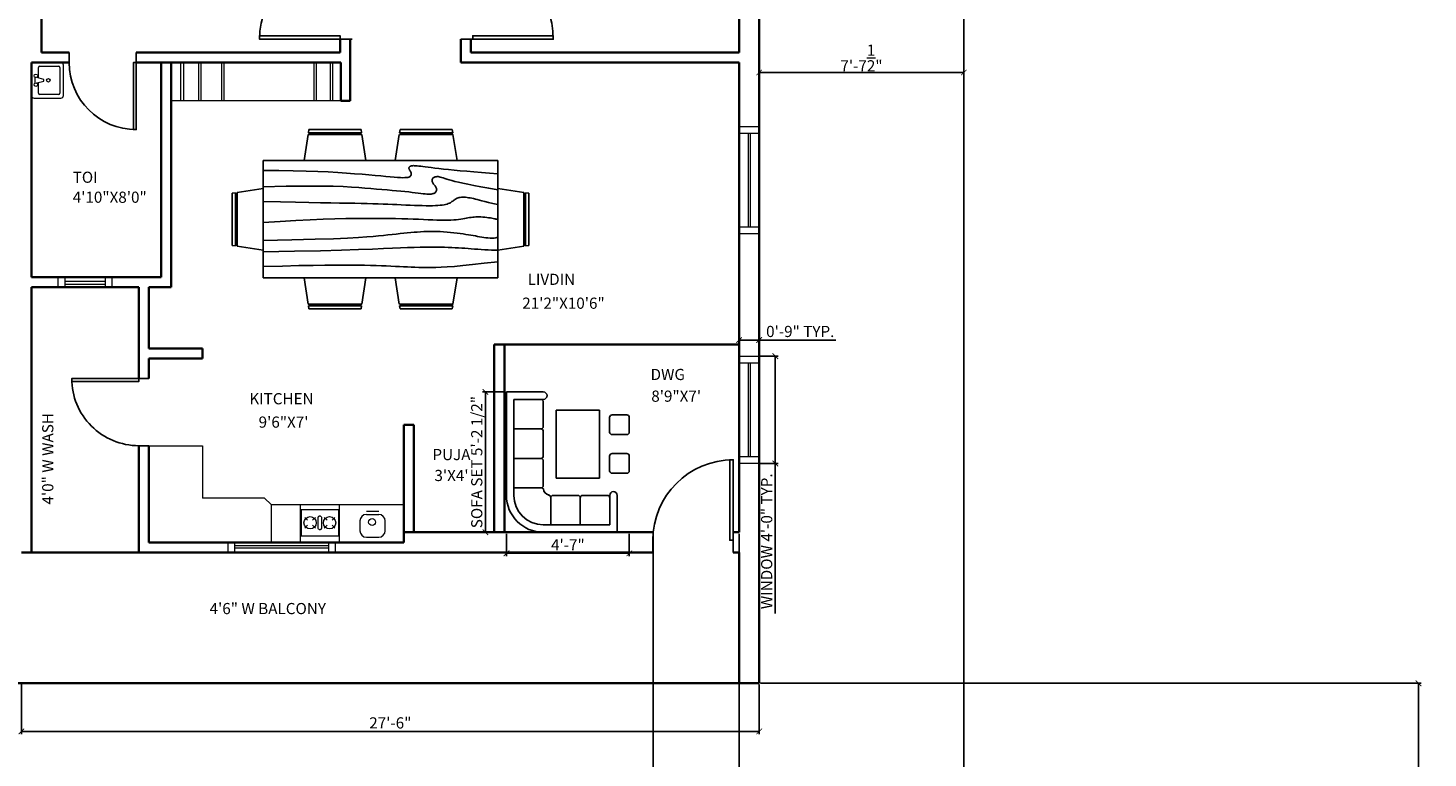
# Model space of a CAD drawing. Units: inches. Extents: x 3283068 to 3284536, y 3240756 to 3241803.
# Tile 18 of 19: x 3283910 to 3284536, y 3241165 to 3241491. Entities that reach past the tile are written whole.
import ezdxf

# ---------------------------------------------------------------- set-up
doc = ezdxf.new("R2010")
doc.units = ezdxf.units.IN
doc.linetypes.add('HIDDEN', pattern=[0.375, 0.25, -0.125])
for name, color, linetype, lineweight in [('A-ANNO-DIMS', 2, 'Continuous', 18), ('A-AREA-IDEN', 7, 'Continuous', 18), ('A-EQPM', 42, 'Continuous', 18), ('A-EQPM-HIDN', 42, 'HIDDEN', 13), ('A-FLOR-CASE', 42, 'Continuous', 18), ('A-FLOR-FIXT', 9, 'Continuous', 18), ('C-PROP', 7, 'Continuous', 25), ('door', 140, 'Continuous', 25), ('furniture', 40, 'Continuous', 18), ('wall', 20, 'Continuous', 35), ('wardrobe', 180, 'Continuous', 18), ('window', 100, 'Continuous', 18)]:
    doc.layers.add(name, color=color, linetype=linetype, lineweight=lineweight)
for name, color, linetype in [('HATCH', 8, 'Continuous'), ('NOI THAT', 42, 'Continuous'), ('NOITHAT', 21, 'Continuous')]:
    doc.layers.add(name, color=color, linetype=linetype)
doc.styles.get("Standard").update_dxf_attribs({"font": 'arial.ttf'})
doc.dimstyles.new('ISO-25', dxfattribs={"dimtxt": 5, "dimasz": 2.5, "dimexe": 1.25, "dimexo": 0.625, "dimtad": 1, "dimlunit": 4, "dimtxsty": 'Standard', "dimblk": 'ARCHTICK', "dimcen": 2.5, "dimadec": 0, "dimazin": 0, "dimtfac": 1, "dimtmove": 0, "dimatfit": 3, "dimfxl": 1, "dimarcsym": 0})

# ---------------------------------------------------------------- blocks, each defined once
blk = doc.blocks.new('*U6')
for p, q in [((0, 0), (0, -6)), ((-40, 0), (-40, -6))]:
    blk.add_line(p, q)
blk.add_lwpolyline([(0, 0), (0, 40), (-1.75, 40), (-1.75, 0)], close=True)
blk.add_arc((0, 0), 40, 90, 180)
blk = doc.blocks.new('*U5')
for p, q in [((-40, 0), (-40, 6)), ((0, 0), (0, 6))]:
    blk.add_line(p, q)
blk.add_lwpolyline([(0, 0), (0, -40), (-1.75, -40), (-1.75, 0)], close=True)
blk.add_arc((0, 0), 40, 180, 270)
blk = doc.blocks.new('*U7')
for p, q in [((0, 0), (0, 6)), ((40, 0), (40, 6))]:
    blk.add_line(p, q)
blk.add_lwpolyline([(0, 0), (0, -40), (1.75, -40), (1.75, 0)], close=True)
blk.add_arc((0, 0), 40, 270, 0)
blk = doc.blocks.new('*U8')
for p, q in [((0, 0), (0, -6)), ((40, 0), (40, -6))]:
    blk.add_line(p, q)
blk.add_lwpolyline([(0, 0), (0, 40), (1.75, 40), (1.75, 0)], close=True)
blk.add_arc((0, 0), 40, 0, 90)
blk = doc.blocks.new('A$C78170A85')
at = {"layer": 'HATCH'}
for points in [[(171.5, 767.4), (258.6, 767), (337.5, 765.8), (408.9, 764), (473.5, 761.7), (532, 759), (585.1, 755.9), (633.5, 752.7), (677.8, 749.3), (718.8, 745.9), (756.5, 742.6), (790.9, 739.5), (822.2, 736.5), (850.3, 733.8), (875.4, 731.5), (897.3, 729.6), (916.3, 728.2), (932.4, 727.4), (945.8, 727.1), (956.7, 727.2), (965.6, 727.9), (972.6, 728.9), (978.1, 730.4), (982.3, 732.1), (985.5, 734.3), (988, 736.6), (989.8, 739.3), (991.1, 742.1), (991.7, 745), (991.9, 748), (991.7, 751), (991, 753.9), (990, 756.8), (988.8, 759.6), (987.3, 762.2), (985.8, 764.7), (984.2, 767.2), (982.7, 769.5), (981.4, 771.9), (980.3, 774.1), (979.5, 776.4), (979.2, 778.6), (979.2, 780.9), (979.7, 783), (980.6, 785), (982, 786.9), (983.7, 788.7), (985.9, 790.2), (988.5, 791.4), (991.6, 792.4), (995.2, 793.1), (999.4, 793.6), (1004.3, 793.7), (1010.1, 793.6), (1016.9, 793.1), (1024.7, 792.4), (1033.7, 791.4), (1043.9, 790.2), (1055.7, 788.6), (1069.2, 786.9), (1084.6, 784.9), (1102.1, 782.6), (1122, 780.2), (1144.5, 777.6), (1169.9, 774.9), (1198.1, 772), (1229.4, 769), (1263.4, 765.9), (1300.1, 762.7), (1339.4, 759.4), (1381.1, 756.1), (1425.2, 752.7), (1471.5, 749.3)], [(171.5, 677.1), (298.3, 679.7), (403.1, 680.8), (488.9, 680.7), (558.5, 679.5), (615, 677.6), (661.2, 675.2), (700.3, 672.4), (735, 669.6), (767.9, 666.8), (799.4, 664.2), (829.5, 661.7), (858.1, 659.2), (885.2, 656.9), (910.7, 654.5), (934.7, 652.3), (956.9, 650), (977.5, 647.8), (996.5, 645.6), (1013.9, 643.5), (1029.7, 641.5), (1044.1, 639.8), (1057, 638.4), (1068.6, 637.2), (1078.8, 636.5), (1087.8, 636.1), (1095.6, 636.2), (1102.4, 636.6), (1108.2, 637.4), (1113.1, 638.6), (1117.3, 640.1), (1120.9, 641.9), (1124, 644), (1126.6, 646.4), (1128.7, 649), (1130.4, 651.9), (1131.7, 654.9), (1132.4, 658.1), (1132.6, 661.3), (1132.3, 664.7), (1131.5, 668.1), (1130.1, 671.4), (1128.2, 674.8), (1126, 678.2), (1123.6, 681.6), (1121, 685), (1118.4, 688.4), (1115.8, 691.8), (1113.4, 695.1), (1111.3, 698.5), (1109.5, 701.9), (1108.2, 705.2), (1107.2, 708.5), (1106.8, 711.7), (1106.9, 714.8), (1107.6, 717.8), (1108.9, 720.7), (1110.9, 723.5), (1113.6, 726), (1116.9, 728.2), (1120.8, 730.1), (1125.1, 731.6), (1129.9, 732.6), (1135, 733), (1140.5, 732.8), (1146.3, 731.8), (1152.7, 730.3), (1159.9, 728.2), (1168.1, 725.5), (1177.6, 722.4), (1188.6, 718.9), (1201.5, 715.1), (1216.5, 710.9), (1233.8, 706.6), (1254.1, 701.9), (1277.9, 696.7), (1305.9, 690.9), (1338.7, 684.4), (1376.8, 677), (1420.9, 668.6), (1471.5, 659)], [(171.5, 595.8), (266.9, 592.9), (350.8, 590.6), (424.4, 588.9), (488.8, 587.7), (545.3, 586.9), (594.9, 586.3), (639, 585.8), (678.6, 585.3), (714.8, 584.7), (748.2, 583.9), (779.2, 583.1), (808.2, 582.1), (835.5, 581.1), (861.6, 580), (886.9, 578.9), (911.8, 577.8), (936.6, 576.7), (961.2, 575.6), (985.3, 574.6), (1008.9, 573.6), (1031.5, 572.9), (1053.1, 572.3), (1073.5, 571.9), (1092.4, 571.8), (1109.6, 571.9), (1125.2, 572.3), (1139.3, 573), (1152, 574), (1163.3, 575.3), (1173.4, 576.8), (1182.3, 578.7), (1190.2, 580.8), (1197, 583.2), (1203, 585.8), (1208.4, 588.6), (1213.1, 591.5), (1217.4, 594.5), (1221.5, 597.5), (1225.4, 600.5), (1229.3, 603.4), (1233.3, 606.1), (1237.5, 608.7), (1242, 611), (1246.8, 613.1), (1251.9, 615), (1257.4, 616.5), (1263.4, 617.6), (1269.9, 618.4), (1277, 618.8), (1284.5, 618.7), (1292.5, 618.3), (1300.9, 617.5), (1309.7, 616.3), (1318.8, 614.8), (1328.1, 613), (1337.6, 610.9), (1347.4, 608.5), (1357.9, 605.7), (1369.8, 602.5), (1383.7, 598.8), (1400.2, 594.6), (1419.9, 589.7), (1443.5, 584.1), (1471.5, 577.8)], [(171.5, 478.5), (265.6, 484.6), (351.7, 489.6), (430.6, 493.6), (502.7, 496.6), (568.7, 498.8), (629.2, 500.4), (684.7, 501.3), (735.8, 501.8), (783, 501.9), (826.7, 501.7), (867.2, 501.3), (904.8, 500.6), (939.8, 499.7), (972.5, 498.7), (1003.2, 497.6), (1032.2, 496.5), (1059.7, 495.4), (1085.8, 494.3), (1110.4, 493.4), (1133.6, 492.6), (1155.2, 492), (1175.4, 491.7), (1194.1, 491.7), (1211.2, 492), (1226.8, 492.8), (1241.1, 493.9), (1254, 495.3), (1266, 496.9), (1277, 498.7), (1287.2, 500.5), (1296.8, 502.3), (1306, 504.1), (1314.9, 505.7), (1323.7, 507.1), (1332.3, 508.3), (1341, 509.3), (1349.8, 510), (1358.9, 510.4), (1368.3, 510.4), (1378.2, 510.1), (1388.6, 509.3), (1399.3, 508.2), (1409.9, 506.9), (1420.3, 505.4), (1430, 503.8), (1438.9, 502.2), (1446.5, 500.8), (1452.7, 499.5), (1457.3, 498.5), (1460.4, 497.8), (1462.6, 497.3), (1464.1, 496.9), (1465.4, 496.7), (1466.8, 496.6), (1468.7, 496.5), (1471.5, 496.5)], [(171.5, 379.2), (330.7, 382.5), (458.9, 385.9), (560.3, 389.2), (639, 392.5), (699.2, 395.7), (745, 398.8), (780.7, 401.9), (810.2, 404.7), (837.3, 407.5), (862.5, 410.1), (886.3, 412.6), (908.7, 414.9), (929.9, 417.1), (950.2, 419.1), (969.7, 421), (988.5, 422.8), (1007, 424.4), (1025.1, 425.9), (1043, 427.1), (1060.8, 428.1), (1078.6, 428.8), (1096.5, 429.1), (1114.6, 429.2), (1133, 428.8), (1151.8, 428.1), (1170.8, 426.9), (1189.9, 425.5), (1208.8, 423.7), (1227.3, 421.8), (1245.3, 419.7), (1262.6, 417.5), (1278.9, 415.3), (1294.2, 413), (1308.5, 410.8), (1321.9, 408.5), (1334.7, 406.3), (1346.9, 404.2), (1358.8, 402.1), (1370.4, 400), (1382, 398), (1393.6, 396.1), (1405.2, 394.4), (1416.7, 393), (1428.2, 392.2), (1439.4, 392.1), (1450.5, 392.8), (1461.2, 394.4), (1471.5, 397.2)], [(171.5, 316), (344.8, 319.3), (488.1, 322.7), (605.2, 325.9), (699.8, 328.9), (776, 331.8), (837.4, 334.4), (887.9, 336.6), (931.4, 338.5), (971, 340), (1007.5, 341.1), (1041.3, 341.9), (1072.4, 342.3), (1101.2, 342.5), (1127.7, 342.4), (1152.3, 342), (1175.1, 341.6), (1196.4, 340.9), (1216.4, 340.2), (1235.3, 339.3), (1253.5, 338.3), (1271.3, 337.2), (1288.7, 335.9), (1306.3, 334.6), (1324.1, 333.3), (1342.4, 331.8), (1361.1, 330.4), (1380, 329), (1398.9, 327.7), (1417.7, 326.6), (1436.2, 325.8), (1454.2, 325.2), (1471.5, 325)], [(171.5, 234.7), (278.3, 237.7), (369.5, 239.9), (447.2, 241.5), (513.2, 242.4), (569.3, 242.9), (617.5, 243), (659.5, 242.7), (697.4, 242.2), (732.7, 241.6), (765.7, 240.9), (796.8, 240), (825.9, 239), (853.4, 238), (879.3, 237), (903.7, 235.8), (926.9, 234.7), (948.9, 233.6), (970.2, 232.5), (991.1, 231.5), (1012, 230.7), (1033.1, 230), (1055, 229.5), (1077.9, 229.3), (1102.1, 229.5), (1128.4, 230), (1157.6, 231), (1191.3, 232.9), (1230.7, 235.8), (1277.1, 239.9), (1331.8, 245.4), (1396.2, 252.7), (1471.5, 261.8)]]:
    blk.add_lwpolyline(points, dxfattribs=at)
at = {"layer": 'NOI THAT'}
for p, q in [((420.1, 966), (397.5, 821.5)), ((420.1, 966), (717.5, 966)), ((424.3, 993.1), (421.5, 975)), ((716.1, 975), (421.5, 975)), ((424.3, 993.1), (713.2, 993.1)), ((716, 975), (713.2, 993.1)), ((740, 821.5), (717.4, 966)), ((925.6, 966), (903.1, 821.5)), ((925.7, 966), (1223.1, 966)), ((929.9, 993.1), (927, 975)), ((1221.6, 975), (927.1, 975)), ((929.9, 993.1), (1218.8, 993.1)), ((1221.6, 975), (1218.8, 993.1)), ((1245.6, 821.5), (1223, 966)), ((1471.5, 821.5), (171.5, 821.5)), ((171.5, 821.5), (171.5, 171.5)), ((1471.5, 171.5), (1471.5, 821.5)), ((0, 641), (18, 643.8)), ((0, 641), (0, 352.1)), ((18.1, 349.2), (18.1, 643.7)), ((27.1, 645.2), (171.6, 667.8)), ((27.1, 645.1), (27.1, 347.8)), ((1616, 645.2), (1471.5, 667.8)), ((1616, 645.1), (1616, 347.8)), ((1643.1, 641), (1625, 643.8)), ((1625, 349.2), (1625, 643.7)), ((1643.1, 641), (1643.1, 352.1)), ((18.1, 349.3), (0, 352.1)), ((171.6, 325.3), (27.1, 347.8)), ((1471.5, 325.3), (1616, 347.8)), ((1625, 349.3), (1643.1, 352.1)), ((420.1, 27.1), (397.5, 171.6)), ((740, 171.6), (717.4, 27.1)), ((925.6, 27.1), (903.1, 171.6)), ((1245.6, 171.6), (1223, 27.1)), ((420.1, 27.1), (717.5, 27.1)), ((716.1, 18.1), (421.5, 18.1)), ((424.3, 0), (421.5, 18)), ((424.3, 0), (713.2, 0)), ((716, 18.1), (713.2, 0)), ((925.7, 27.1), (1223.1, 27.1)), ((929.9, 0), (927, 18)), ((1221.6, 18.1), (927.1, 18.1)), ((929.9, 0), (1218.8, 0)), ((1221.6, 18.1), (1218.8, 0))]:
    blk.add_line(p, q, dxfattribs=at)
at = {"layer": 'NOI THAT', "ltscale": 20}
blk.add_line((171.5, 171.5), (1471.5, 171.5), dxfattribs=at)
blk = doc.blocks.new('A$C066B3FC2')
at = {"layer": 'NOITHAT'}
for p, q in [((750, 2498), (2850, 2498)), ((750, 2348), (2700, 2348)), ((900, 1786), (900, 2348)), ((1500, 1798), (1500, 2348)), ((1500, 1798), (1500, 2348)), ((2100, 1798), (2100, 2348)), ((2700, 1748), (2700, 2348)), ((2850, 1748), (2850, 2498)), ((0, 248), (0, 1748)), ((150, 398), (150, 1748)), ((950, 1748), (1450, 1748)), ((1550, 1748), (2050, 1748)), ((2150, 1748), (2650, 1748)), ((707, 1598), (150, 1598)), ((750, 1048), (750, 1548)), ((2480, 1489), (1098, 1489)), ((1098, 1489), (1098, 606)), ((2480, 606), (2480, 1489)), ((700, 998), (150, 998)), ((750, 448), (750, 948)), ((1098, 606), (2480, 606)), ((750, 398), (150, 398)), ((1200, 50), (1200, 350)), ((1250, 400), (1550, 400)), ((1600, 350), (1600, 50)), ((1985, 50), (1985, 350)), ((2035, 400), (2335, 400)), ((2385, 350), (2385, 50)), ((750, 248), (0, 248)), ((1550, 0), (1250, 0)), ((2335, 0), (2035, 0))]:
    blk.add_line(p, q, dxfattribs=at)
for centre, radius, start, end in [((750, 1748), 750, 90, 180), ((750, 1748), 600, 90, 180), ((900, 1598), 150, 97.3131, 166.7789), ((850, 1786), 50, 308.1793, 0), ((950, 1798), 50, 180, 270), ((1450, 1798), 50, 270, 0), ((1450, 1798), 50, 270, 0), ((1550, 1798), 50, 180, 270), ((1550, 1798), 50, 180, 270), ((2050, 1798), 50, 270, 0), ((2150, 1798), 50, 180, 270), ((2650, 1798), 50, 270, 0), ((2775, 1748), 75, 180, 0), ((700, 1548), 50, 0, 90), ((707, 1648), 50, 270, 349.3159), ((700, 1048), 50, 270, 0), ((700, 948), 50, 0, 90), ((700, 448), 50, 270, 0), ((750, 323), 75, 270, 90), ((1250, 350), 50, 90, 180), ((1550, 350), 50, 0, 90), ((2035, 350), 50, 90, 180), ((2335, 350), 50, 0, 90), ((1250, 50), 50, 180, 270), ((1550, 50), 50, 270, 0), ((2035, 50), 50, 180, 270), ((2335, 50), 50, 270, 0)]:
    blk.add_arc(centre, radius, start, end, dxfattribs=at)
blk = doc.blocks.new('_ArchTick')
at = {"color": 0, "linetype": 'ByBlock', "const_width": 0.15}
blk.add_lwpolyline([(-0.5, -0.5), (0.5, 0.5)], dxfattribs=at)
blk = doc.blocks.new('*D28')
at = {"layer": 'A-ANNO-DIMS', "color": 0, "lineweight": -2, "transparency": 16777216}
for p, q in [((3283906.59, 3241197.48), (3283906.59, 3241175.31)), ((3284236.59, 3241197.48), (3284236.59, 3241175.31)), ((3283906.59, 3241176.56), (3284236.59, 3241176.56))]:
    blk.add_line(p, q, dxfattribs=at)
at = {"layer": 'Defpoints', "color": 0, "transparency": 16777216}
for p in [(3283906.59, 3241198.1), (3284236.59, 3241198.1), (3284236.59, 3241176.56)]:
    blk.add_point(p, dxfattribs=at)
at = {"layer": 'A-ANNO-DIMS', "color": 0, "lineweight": -2, "transparency": 16777216, "xscale": 2.5, "yscale": 2.5, "zscale": 2.5, "rotation": 180}
blk.add_blockref('_ArchTick', (3283906.59, 3241176.56), dxfattribs=at)
at = {"layer": 'A-ANNO-DIMS', "color": 0, "lineweight": -2, "transparency": 16777216, "xscale": 2.5, "yscale": 2.5, "zscale": 2.5}
blk.add_blockref('_ArchTick', (3284236.59, 3241176.56), dxfattribs=at)
at = {"layer": 'A-ANNO-DIMS', "color": 0, "transparency": 16777216, "insert": (3284071.59, 3241179.74), "char_height": 5, "attachment_point": 5}
blk.add_mtext('27\'-6"', dxfattribs=at)
blk = doc.blocks.new('*D35')
at = {"layer": 'A-ANNO-DIMS', "color": 0, "lineweight": -2, "transparency": 16777216}
for p, q in [((3284236.59, 3241464.98), (3284236.59, 3241472.39)), ((3284236.59, 3241471.14), (3284328.09, 3241471.14)), ((3284328.09, 3241464.98), (3284328.09, 3241472.39))]:
    blk.add_line(p, q, dxfattribs=at)
at = {"layer": 'Defpoints', "color": 0, "transparency": 16777216}
for p in [(3284328.09, 3241471.14), (3284236.59, 3241464.36), (3284328.09, 3241464.36)]:
    blk.add_point(p, dxfattribs=at)
at = {"layer": 'A-ANNO-DIMS', "color": 0, "lineweight": -2, "transparency": 16777216, "xscale": 2.5, "yscale": 2.5, "zscale": 2.5, "rotation": 180}
blk.add_blockref('_ArchTick', (3284236.59, 3241471.14), dxfattribs=at)
at = {"layer": 'A-ANNO-DIMS', "color": 0, "lineweight": -2, "transparency": 16777216, "xscale": 2.5, "yscale": 2.5, "zscale": 2.5}
blk.add_blockref('_ArchTick', (3284328.09, 3241471.14), dxfattribs=at)
at = {"layer": 'A-ANNO-DIMS', "color": 0, "transparency": 16777216, "insert": (3284282.34, 3241477.62), "char_height": 5, "attachment_point": 5}
blk.add_mtext('7\'-7{\\H1x;\\S1/2;}"', dxfattribs=at)
blk = doc.blocks.new('WIN-48IN-9IN-WALL')
for p, q in [((0, 9), (48, 9)), ((0, 0), (0, 9)), ((3, 0), (3, 9)), ((45, 9), (45, 0)), ((48, 9), (48, 0)), ((48, 0), (0, 0)), ((3, 5), (45, 5)), ((3, 4), (45, 4))]:
    blk.add_line(p, q)
blk = doc.blocks.new('WIN-24IN-4_5IN-WALL')
for p, q in [((0, 4.5), (24, 4.5)), ((0, 0), (0, 4.5)), ((24, 0), (0, 0)), ((3, 0), (3, 4.5)), ((3, 2.73), (21, 2.73)), ((3, 1.44), (21, 1.44)), ((21, 4.5), (21, 0)), ((24, 4.5), (24, 0))]:
    blk.add_line(p, q)
blk = doc.blocks.new('LAVATORY-COMPACT')
for p, q in [((0, 14.71), (0, 1.19)), ((13.12, 15.9), (1.19, 15.9)), ((3.18, 8.94), (3.18, 13.71)), ((3.78, 14.31), (12.12, 14.31)), ((12.72, 13.71), (12.72, 2.19)), ((14.31, 1.19), (14.31, 14.71)), ((1.59, 6.76), (1.59, 9.14)), ((5.56, 8.35), (2.38, 9.14)), ((2.38, 6.76), (5.56, 7.55)), ((3.18, 2.19), (3.18, 6.96)), ((5.56, 7.55), (5.56, 8.35)), ((1.19, 0), (13.12, 0)), ((12.12, 1.59), (3.78, 1.59))]:
    blk.add_line(p, q)
for centre in [(1.99, 9.94), (1.99, 5.96), (7.55, 7.95)]:
    blk.add_circle(centre, 0.795)
for centre, radius, start, end in [((1.19, 14.71), 1.19, 90, 180), ((3.78, 13.71), 0.596, 90, 180), ((12.12, 13.71), 0.596, 0, 90), ((13.12, 14.71), 1.19, 0, 90), ((1.19, 1.19), 1.19, 180, 270), ((3.78, 2.19), 0.596, 180, 270), ((12.12, 2.19), 0.596, 270, 0), ((13.12, 1.19), 1.19, 270, 0)]:
    blk.add_arc(centre, radius, start, end)
blk = doc.blocks.new('*D41')
at = {"layer": 'A-ANNO-DIMS', "color": 0, "lineweight": -2, "transparency": 16777216}
for p, q in [((3284237.21, 3241344.34), (3284245.04, 3241344.34)), ((3284243.79, 3241344.34), (3284243.79, 3241296.34)), ((3284237.21, 3241296.34), (3284245.04, 3241296.34)), ((3284243.79, 3241296.34), (3284243.79, 3241229.32))]:
    blk.add_line(p, q, dxfattribs=at)
at = {"layer": 'Defpoints', "color": 0, "transparency": 16777216}
for p in [(3284236.59, 3241344.34), (3284236.59, 3241296.34), (3284243.79, 3241296.34)]:
    blk.add_point(p, dxfattribs=at)
at = {"layer": 'A-ANNO-DIMS', "color": 0, "lineweight": -2, "transparency": 16777216, "xscale": 2.5, "yscale": 2.5, "zscale": 2.5}
for p, rotation in [((3284243.79, 3241344.34), 90), ((3284243.79, 3241296.34), 270)]:
    blk.add_blockref('_ArchTick', p, dxfattribs=dict(at, rotation=rotation))
at = {"layer": 'A-ANNO-DIMS', "color": 0, "transparency": 16777216, "insert": (3284240.58, 3241261.58), "char_height": 5, "attachment_point": 5, "rotation": 90}
blk.add_mtext('WINDOW 4\'-0" TYP.', dxfattribs=at)
blk = doc.blocks.new('*D42')
at = {"layer": 'A-ANNO-DIMS', "color": 0, "lineweight": -2, "transparency": 16777216}
for p, q in [((3284227.59, 3241344.97), (3284227.59, 3241352.79)), ((3284236.59, 3241344.97), (3284236.59, 3241352.79)), ((3284227.59, 3241351.54), (3284236.59, 3241351.54)), ((3284236.59, 3241351.54), (3284270.82, 3241351.54))]:
    blk.add_line(p, q, dxfattribs=at)
at = {"layer": 'Defpoints', "color": 0, "transparency": 16777216}
for p in [(3284236.59, 3241351.54), (3284227.59, 3241344.34), (3284236.59, 3241344.34)]:
    blk.add_point(p, dxfattribs=at)
at = {"layer": 'A-ANNO-DIMS', "color": 0, "lineweight": -2, "transparency": 16777216, "xscale": 2.5, "yscale": 2.5, "zscale": 2.5, "rotation": 180}
blk.add_blockref('_ArchTick', (3284227.59, 3241351.54), dxfattribs=at)
at = {"layer": 'A-ANNO-DIMS', "color": 0, "lineweight": -2, "transparency": 16777216, "xscale": 2.5, "yscale": 2.5, "zscale": 2.5}
blk.add_blockref('_ArchTick', (3284236.59, 3241351.54), dxfattribs=at)
at = {"layer": 'A-ANNO-DIMS', "color": 0, "transparency": 16777216, "insert": (3284254.95, 3241354.72), "char_height": 5, "attachment_point": 5}
blk.add_mtext('0\'-9" TYP.', dxfattribs=at)
blk = doc.blocks.new('*D59')
at = {"layer": 'A-ANNO-DIMS', "color": 0, "lineweight": -2, "transparency": 16777216}
for p, q in [((3284122.89, 3241328.33), (3284112.86, 3241328.33)), ((3284114.11, 3241265.6), (3284114.11, 3241328.33)), ((3284122.89, 3241265.6), (3284112.86, 3241265.6))]:
    blk.add_line(p, q, dxfattribs=at)
at = {"layer": 'Defpoints', "color": 0, "transparency": 16777216}
for p in [(3284114.11, 3241328.33), (3284123.52, 3241328.33), (3284123.52, 3241265.6)]:
    blk.add_point(p, dxfattribs=at)
at = {"layer": 'A-ANNO-DIMS', "color": 0, "lineweight": -2, "transparency": 16777216, "xscale": 2.5, "yscale": 2.5, "zscale": 2.5}
for p, rotation in [((3284114.11, 3241328.33), 90), ((3284114.11, 3241265.6), 270)]:
    blk.add_blockref('_ArchTick', p, dxfattribs=dict(at, rotation=rotation))
at = {"layer": 'A-ANNO-DIMS', "color": 0, "transparency": 16777216, "insert": (3284110.9, 3241296.97), "char_height": 5, "attachment_point": 5, "rotation": 90}
blk.add_mtext('SOFA SET 5\'-2 1/2"', dxfattribs=at)
blk = doc.blocks.new('*D60')
at = {"layer": 'A-ANNO-DIMS', "color": 0, "lineweight": -2, "transparency": 16777216}
for p, q in [((3284123.52, 3241264.98), (3284123.52, 3241254.94)), ((3284178.49, 3241264.98), (3284178.49, 3241254.94)), ((3284178.49, 3241256.19), (3284123.52, 3241256.19))]:
    blk.add_line(p, q, dxfattribs=at)
at = {"layer": 'Defpoints', "color": 0, "transparency": 16777216}
for p in [(3284123.52, 3241265.6), (3284178.49, 3241265.6), (3284123.52, 3241256.19)]:
    blk.add_point(p, dxfattribs=at)
at = {"layer": 'A-ANNO-DIMS', "color": 0, "lineweight": -2, "transparency": 16777216, "xscale": 2.5, "yscale": 2.5, "zscale": 2.5, "rotation": 180}
blk.add_blockref('_ArchTick', (3284123.52, 3241256.19), dxfattribs=at)
at = {"layer": 'A-ANNO-DIMS', "color": 0, "lineweight": -2, "transparency": 16777216, "xscale": 2.5, "yscale": 2.5, "zscale": 2.5}
blk.add_blockref('_ArchTick', (3284178.49, 3241256.19), dxfattribs=at)
at = {"layer": 'A-ANNO-DIMS', "color": 0, "transparency": 16777216, "insert": (3284151, 3241259.32), "char_height": 5, "attachment_point": 5}
blk.add_mtext('4\'-7"', dxfattribs=at)
blk = doc.blocks.new('*D62')
at = {"layer": 'A-ANNO-DIMS', "color": 0, "lineweight": -2, "transparency": 16777216}
for p, q in [((3284237.21, 3241198.1), (3284532.74, 3241198.1)), ((3284531.49, 3241198.1), (3284531.49, 3241082.6)), ((3284328.71, 3241082.6), (3284532.74, 3241082.6))]:
    blk.add_line(p, q, dxfattribs=at)
at = {"layer": 'Defpoints', "color": 0, "transparency": 16777216}
for p in [(3284236.59, 3241198.1), (3284328.09, 3241082.6), (3284531.49, 3241082.6)]:
    blk.add_point(p, dxfattribs=at)
at = {"layer": 'A-ANNO-DIMS', "color": 0, "lineweight": -2, "transparency": 16777216, "xscale": 2.5, "yscale": 2.5, "zscale": 2.5}
for p, rotation in [((3284531.49, 3241198.1), 90), ((3284531.49, 3241082.6), 270)]:
    blk.add_blockref('_ArchTick', p, dxfattribs=dict(at, rotation=rotation))
at = {"layer": 'A-ANNO-DIMS', "color": 0, "transparency": 16777216, "insert": (3284528.28, 3241140.35), "char_height": 5, "attachment_point": 5, "rotation": 90}
blk.add_mtext('9\'-7 1/2"', dxfattribs=at)
blk = doc.blocks.new('*D63')
at = {"layer": 'A-ANNO-DIMS', "color": 0, "lineweight": -2, "transparency": 16777216}
for p, q in [((3283248.09, 3241083.23), (3283248.09, 3241798.08)), ((3283248.09, 3241796.83), (3284328.09, 3241796.83)), ((3284328.09, 3241083.23), (3284328.09, 3241798.08))]:
    blk.add_line(p, q, dxfattribs=at)
at = {"layer": 'Defpoints', "color": 0, "transparency": 16777216}
for p in [(3284328.09, 3241796.83), (3283248.09, 3241082.6), (3284328.09, 3241082.6)]:
    blk.add_point(p, dxfattribs=at)
at = {"layer": 'A-ANNO-DIMS', "color": 0, "lineweight": -2, "transparency": 16777216, "xscale": 2.5, "yscale": 2.5, "zscale": 2.5, "rotation": 180}
blk.add_blockref('_ArchTick', (3283248.09, 3241796.83), dxfattribs=at)
at = {"layer": 'A-ANNO-DIMS', "color": 0, "lineweight": -2, "transparency": 16777216, "xscale": 2.5, "yscale": 2.5, "zscale": 2.5}
blk.add_blockref('_ArchTick', (3284328.09, 3241796.83), dxfattribs=at)
at = {"layer": 'A-ANNO-DIMS', "color": 0, "transparency": 16777216, "insert": (3283788.09, 3241800.01), "char_height": 5, "attachment_point": 5}
blk.add_mtext('90\'-0"', dxfattribs=at)
blk = doc.blocks.new('*D65')
at = {"layer": 'A-ANNO-DIMS', "color": 0, "lineweight": -2, "transparency": 16777216}
for p, q in [((3284189.18, 3241264.98), (3284189.18, 3240759.03)), ((3284227.59, 3241264.98), (3284227.59, 3240759.03)), ((3284189.18, 3240760.28), (3284227.59, 3240760.28))]:
    blk.add_line(p, q, dxfattribs=at)
at = {"layer": 'Defpoints', "color": 0, "transparency": 16777216}
for p in [(3284189.18, 3241265.6), (3284227.59, 3241265.6), (3284227.59, 3240760.28)]:
    blk.add_point(p, dxfattribs=at)
at = {"layer": 'A-ANNO-DIMS', "color": 0, "lineweight": -2, "transparency": 16777216, "xscale": 2.5, "yscale": 2.5, "zscale": 2.5, "rotation": 180}
blk.add_blockref('_ArchTick', (3284189.18, 3240760.28), dxfattribs=at)
at = {"layer": 'A-ANNO-DIMS', "color": 0, "lineweight": -2, "transparency": 16777216, "xscale": 2.5, "yscale": 2.5, "zscale": 2.5}
blk.add_blockref('_ArchTick', (3284227.59, 3240760.28), dxfattribs=at)
at = {"layer": 'A-ANNO-DIMS', "color": 0, "transparency": 16777216, "insert": (3284208.39, 3240763.49), "char_height": 5, "attachment_point": 5}
blk.add_mtext('3\'-2 1/2"', dxfattribs=at)

msp = doc.modelspace()

# ---------------------------------------------------------------- linework, layer by layer
at = {"layer": 'A-EQPM'}
for p, q in [((3284031.639, 3241275.639), (3284031.639, 3241264.01)), ((3284048.501, 3241275.639), (3284031.639, 3241275.639)), ((3284034.579, 3241270.984), (3284033.345, 3241272.217)), ((3284038.073, 3241272.217), (3284036.84, 3241270.984)), ((3284043.3, 3241270.984), (3284042.067, 3241272.217)), ((3284046.795, 3241272.217), (3284045.562, 3241270.984)), ((3284048.501, 3241264.01), (3284048.501, 3241275.639)), ((3284031.639, 3241264.01), (3284048.501, 3241264.01)), ((3284034.579, 3241268.723), (3284033.345, 3241267.489)), ((3284038.073, 3241267.489), (3284036.84, 3241268.723)), ((3284043.3, 3241268.723), (3284042.067, 3241267.489)), ((3284046.795, 3241267.489), (3284045.562, 3241268.723))]:
    msp.add_line(p, q, dxfattribs=at)
for centre in [(3284035.709, 3241269.853), (3284044.431, 3241269.853)]:
    msp.add_circle(centre, 2.762, dxfattribs=at)
at = {"layer": 'A-EQPM-HIDN'}
for p, q in [((3284039.198, 3241272.15), (3284039.198, 3241267.498)), ((3284040.361, 3241272.731), (3284039.78, 3241272.731)), ((3284040.942, 3241267.498), (3284040.942, 3241272.15)), ((3284039.78, 3241266.917), (3284040.361, 3241266.917))]:
    msp.add_line(p, q, dxfattribs=at)
for centre, start, end in [((3284039.78, 3241272.15), 90, 180), ((3284040.361, 3241272.15), 0, 90), ((3284039.78, 3241267.498), 180, 270), ((3284040.361, 3241267.498), 270, 0)]:
    msp.add_arc(centre, 0.581, start, end, dxfattribs=at)
at = {"layer": 'A-FLOR-CASE'}
for p, q in [((3283963.589, 3241261.102), (3283963.589, 3241304.314)), ((3283963.589, 3241304.271), (3283987.589, 3241304.271)), ((3283987.589, 3241304.271), (3283987.589, 3241280.872)), ((3284015.359, 3241280.872), (3283987.589, 3241280.872)), ((3284018.266, 3241277.964), (3284015.359, 3241280.872)), ((3284018.266, 3241277.964), (3284018.266, 3241261.102)), ((3284018.266, 3241277.964), (3284066.235, 3241277.964)), ((3284031.349, 3241261.102), (3284031.349, 3241277.964)), ((3284048.792, 3241261.102), (3284048.792, 3241277.964)), ((3284066.235, 3241277.964), (3284077.589, 3241277.964)), ((3284077.589, 3241277.964), (3284077.589, 3241261.102)), ((3283997.536, 3241261.102), (3284015.359, 3241261.102)), ((3283999.369, 3241261.102), (3284077.589, 3241261.102))]:
    msp.add_line(p, q, dxfattribs=at)
at = {"layer": 'A-FLOR-FIXT'}
for p, q in [((3284057.972, 3241270.664), (3284057.972, 3241266.303)), ((3284060.88, 3241275.025), (3284066.403, 3241275.025)), ((3284060.88, 3241273.571), (3284066.403, 3241273.571)), ((3284069.311, 3241266.303), (3284069.311, 3241270.664)), ((3284060.88, 3241263.396), (3284066.403, 3241263.396))]:
    msp.add_line(p, q, dxfattribs=at)
msp.add_circle((3284063.447, 3241270.167), 1.548, dxfattribs=at)
for centre, start, end in [((3284060.88, 3241270.664), 90, 180), ((3284066.403, 3241270.664), 0, 90), ((3284060.88, 3241266.303), 180, 270), ((3284066.403, 3241266.303), 270, 0)]:
    msp.add_arc(centre, 2.907, start, end, dxfattribs=at)
at = {"layer": 'C-PROP'}
msp.add_line((3284328.089, 3241730.602), (3284328.089, 3241082.602), dxfattribs=at)
at = {"layer": 'door'}
for p, q in [((3284049.089, 3241485.971), (3284053.589, 3241485.971)), ((3284103.089, 3241485.971), (3284107.589, 3241485.971)), ((3283927.953, 3241475.602), (3283927.953, 3241480.102)), ((3283963.589, 3241334.314), (3283959.089, 3241334.314))]:
    msp.add_line(p, q, dxfattribs=at)
at = {"layer": 'wall'}
for p, q in [((3284236.589, 3241639.102), (3284236.589, 3241198.102)), ((3283915.589, 3241630.102), (3283915.589, 3241480.102)), ((3284227.589, 3241630.102), (3284227.589, 3241480.102)), ((3284049.089, 3241485.971), (3284049.089, 3241480.102)), ((3284053.589, 3241485.971), (3284053.589, 3241475.602)), ((3284103.089, 3241485.971), (3284103.089, 3241475.602)), ((3284107.589, 3241485.971), (3284107.589, 3241480.102)), ((3283915.589, 3241480.102), (3283927.953, 3241480.102)), ((3283957.953, 3241480.102), (3284049.089, 3241480.102)), ((3284107.589, 3241480.102), (3284227.589, 3241480.102)), ((3283911.089, 3241475.602), (3283927.953, 3241475.602)), ((3283911.089, 3241475.602), (3283911.089, 3241379.602)), ((3283911.089, 3241475.602), (3283911.089, 3241379.602)), ((3283957.953, 3241475.602), (3284049.396, 3241475.602)), ((3283969.089, 3241475.602), (3283969.089, 3241379.602)), ((3283973.589, 3241475.602), (3283973.589, 3241375.102)), ((3284049.396, 3241475.602), (3284049.396, 3241458.418)), ((3284053.589, 3241475.602), (3284053.589, 3241465.233)), ((3284053.589, 3241475.602), (3284053.589, 3241458.418)), ((3284103.089, 3241475.602), (3284227.589, 3241475.602)), ((3284227.589, 3241475.602), (3284227.589, 3241265.602)), ((3284049.396, 3241458.418), (3284053.589, 3241458.418)), ((3283911.089, 3241379.602), (3283969.089, 3241379.602)), ((3283911.089, 3241375.102), (3283959.089, 3241375.102)), ((3283911.089, 3241375.102), (3283911.089, 3241256.602)), ((3283959.089, 3241375.102), (3283959.089, 3241334.314)), ((3283963.589, 3241375.102), (3283963.589, 3241347.72)), ((3283963.589, 3241375.102), (3283973.589, 3241375.102)), ((3283963.589, 3241347.72), (3283987.589, 3241347.72)), ((3283987.589, 3241347.72), (3283987.589, 3241343.22)), ((3284118.089, 3241349.602), (3284227.589, 3241349.602)), ((3284118.089, 3241349.602), (3284118.089, 3241265.602)), ((3284122.589, 3241349.602), (3284122.589, 3241265.602)), ((3283963.589, 3241343.22), (3283987.589, 3241343.22)), ((3283963.589, 3241343.22), (3283963.589, 3241334.314)), ((3284077.589, 3241313.602), (3284077.589, 3241265.602)), ((3284077.589, 3241313.602), (3284082.089, 3241313.602)), ((3284082.089, 3241313.602), (3284082.089, 3241265.602)), ((3283959.089, 3241304.314), (3283959.089, 3241256.602)), ((3283963.589, 3241304.314), (3283963.589, 3241261.102)), ((3284077.589, 3241265.602), (3284189.185, 3241265.602)), ((3284077.589, 3241265.602), (3284077.589, 3241261.102)), ((3284225.004, 3241265.602), (3284227.589, 3241265.602)), ((3284077.589, 3241261.102), (3283963.589, 3241261.102)), ((3283906.589, 3241256.602), (3284189.004, 3241256.602)), ((3284225.004, 3241256.602), (3284227.589, 3241256.602)), ((3284227.589, 3241256.602), (3284227.589, 3241198.102)), ((3283339.589, 3241198.102), (3284236.589, 3241198.102))]:
    msp.add_line(p, q, dxfattribs=at)
at = {"layer": 'wardrobe'}
for p, q in [((3283977.751, 3241475.602), (3283977.751, 3241458.418)), ((3283979.126, 3241475.602), (3283979.126, 3241458.418)), ((3283985.845, 3241475.602), (3283985.845, 3241458.418)), ((3283986.841, 3241475.602), (3283986.841, 3241458.418)), ((3283996.109, 3241475.602), (3283996.109, 3241458.418)), ((3283997.097, 3241475.602), (3283997.097, 3241458.418)), ((3284037.415, 3241475.602), (3284037.415, 3241458.418)), ((3284038.4, 3241475.602), (3284038.4, 3241458.418)), ((3284044.751, 3241475.602), (3284044.751, 3241458.418)), ((3284045.777, 3241475.602), (3284045.777, 3241458.418))]:
    msp.add_line(p, q, dxfattribs=at)
msp.add_lwpolyline([(3283973.589, 3241475.602), (3284049.396, 3241475.602), (3284049.396, 3241458.418), (3283973.589, 3241458.418)], close=True, dxfattribs=at)
at = {"layer": 'window'}
for p, q in [((3283998.986, 3241261.102), (3284046.986, 3241261.102)), ((3283998.986, 3241256.602), (3283998.986, 3241261.102)), ((3284001.986, 3241256.602), (3284001.986, 3241261.102)), ((3284001.986, 3241259.691), (3284043.986, 3241259.691)), ((3284001.986, 3241258.691), (3284043.986, 3241258.691)), ((3284043.986, 3241261.102), (3284043.986, 3241256.602)), ((3284046.986, 3241261.102), (3284046.986, 3241256.602)), ((3284046.986, 3241256.602), (3283998.986, 3241256.602))]:
    msp.add_line(p, q, dxfattribs=at)

# ---------------------------------------------------------------- block references
at = {"layer": 'A-FLOR-FIXT'}
msp.add_blockref('LAVATORY-COMPACT', (3283911.079, 3241459.704), dxfattribs=at)
at = {"layer": 'door'}
for name, p, xscale, yscale, zscale, rotation in [('*U5', (3284049.089, 3241485.971), 0.9, 0.9, 0.9, 270), ('*U6', (3284108.489, 3241485.971), 0.9, 0.9, 0.9, 270), ('*U8', (3283957.953, 3241475.602), 0.75, 0.75, 0.75, 180), ('*U7', (3283959.089, 3241334.314), 0.75, 0.75, 0.75, 270)]:
    msp.add_blockref(name, p, dxfattribs=dict(at, xscale=xscale, yscale=yscale, zscale=zscale, rotation=rotation))
at = {"layer": 'door', "xscale": 0.9, "yscale": 0.9, "zscale": 0.9}
msp.add_blockref('*U6', (3284225.004, 3241262.002), dxfattribs=at)
at = {"layer": 'furniture', "xscale": 0.0807042311318891, "yscale": 0.0807042311318891, "zscale": 0.0807042311318891}
msp.add_blockref('A$C78170A85', (3284000.917, 3241365.436), dxfattribs=at)
at = {"layer": 'furniture', "xscale": 0.0220088795959633, "yscale": 0.0220088795959633, "zscale": 0.0220088795959633, "rotation": 90}
msp.add_blockref('A$C066B3FC2', (3284178.492, 3241265.602), dxfattribs=at)
at = {"layer": 'window'}
for p, rotation in [((3284227.589, 3241447.006), 270.0000000012753), ((3284227.589, 3241344.344), 270.0000000006712)]:
    msp.add_blockref('WIN-48IN-9IN-WALL', p, dxfattribs=dict(at, rotation=rotation))
msp.add_blockref('WIN-24IN-4_5IN-WALL', (3283923.09, 3241375.102), dxfattribs=at)

# ---------------------------------------------------------------- texts
at = {"layer": 'A-AREA-IDEN'}
for s, p in [('TOI', (3283929.528, 3241421.811)), ('4\'10"X8\'0"', (3283929.528, 3241412.881)), ('LIVDIN', (3284133.005, 3241376.182)), ('21\'2"X10\'6"', (3284130.591, 3241365.501)), ('DWG', (3284187.991, 3241333.653)), ('KITCHEN', (3284008.521, 3241322.803)), ('8\'9"X7\'', (3284188.311, 3241323.951)), ('9\'6"X7\'', (3284012.688, 3241312.353)), ('PUJA', (3284090.421, 3241297.844)), ("3'X4'", (3284091.322, 3241288.494))]:
    msp.add_text(s, height=5, dxfattribs=at).set_placement(p)
at = {"layer": 'A-AREA-IDEN', "insert": (3283915.863, 3241278), "char_height": 5, "attachment_point": 1, "rotation": 90}
msp.add_mtext_dynamic_manual_height_columns('4\'0" W WASH', width=85.09051, gutter_width=12.5, heights=[0], dxfattribs=at)
at = {"layer": 'A-AREA-IDEN', "insert": (3283990.751, 3241233.997), "char_height": 5, "attachment_point": 1}
msp.add_mtext_dynamic_manual_height_columns('4\'6" W BALCONY', width=85.09051, gutter_width=12.5, heights=[0], dxfattribs=at)

# ---------------------------------------------------------------- dimensions: what is measured, and where the dimension line sits
at = {"layer": 'A-ANNO-DIMS'}
for base, p1, p2, override, picture, middle in [((3284328.089, 3241796.827), (3283248.089, 3241082.602), (3284328.089, 3241082.602), {"dimdec": 1, "dimlfac": 1, "dimrnd": 0, "dimzin": 1, "dimdsep": 46, "dimlunit": 4, "dimfrac": 2}, '*D63', (3283788.089, 3241800.005)), ((3284328.089, 3241471.137), (3284236.589, 3241464.358), (3284328.089, 3241464.358), {"dimclrd": 0, "dimclre": 0, "dimclrt": 0}, '*D35', (3284282.339, 3241477.615)), ((3284227.589, 3240760.281), (3284189.185, 3241265.602), (3284227.589, 3241265.602), {"dimdec": 1, "dimlfac": 1, "dimrnd": 0, "dimzin": 1, "dimdsep": 46, "dimlunit": 4, "dimfrac": 2}, '*D65', (3284208.387, 3240763.493)), ((3284236.589, 3241176.561), (3283906.589, 3241198.102), (3284236.589, 3241198.102), {"dimclrd": 0, "dimclre": 0, "dimclrt": 0, "dimtmove": 1}, '*D28', (3284071.589, 3241179.739))]:
    dim = msp.add_linear_dim(base=base, p1=p1, p2=p2, dimstyle='ISO-25', override=override, dxfattribs=at)
    dim.commit()
    dim.dimension.update_dxf_attribs({"geometry": picture, "text_midpoint": middle})
dim = msp.add_linear_dim(base=(3284236.589, 3241351.543), p1=(3284227.589, 3241344.343), p2=(3284236.589, 3241344.343), text='<> TYP.', dimstyle='ISO-25', override={"dimdec": 1, "dimlfac": 1, "dimrnd": 0, "dimzin": 1, "dimdsep": 46, "dimlunit": 4, "dimfrac": 2}, dxfattribs=at)
dim.commit()
dim.dimension.update_dxf_attribs({"geometry": '*D42', "text_midpoint": (3284254.953, 3241354.721)})
for base, p1, p2, angle, text, picture, middle in [((3284243.789, 3241296.343), (3284236.589, 3241344.343), (3284236.589, 3241296.343), 270, 'WINDOW <> TYP.', '*D41', (3284240.577, 3241261.583)), ((3284114.109, 3241328.328), (3284123.518, 3241265.602), (3284123.518, 3241328.328), 90, 'SOFA SET <>', '*D59', (3284110.897, 3241296.965))]:
    dim = msp.add_linear_dim(base=base, p1=p1, p2=p2, angle=angle, text=text, dimstyle='ISO-25', override={"dimdec": 1, "dimlfac": 1, "dimrnd": 0, "dimzin": 1, "dimdsep": 46, "dimlunit": 4, "dimfrac": 2}, dxfattribs=at)
    dim.commit()
    dim.dimension.update_dxf_attribs({"geometry": picture, "text_midpoint": middle})
for base, p1, p2, angle, picture, middle in [((3284123.518, 3241256.194), (3284178.492, 3241265.602), (3284123.518, 3241265.602), 180, '*D60', (3284151.005, 3241259.319)), ((3284531.489, 3241082.602), (3284236.589, 3241198.102), (3284328.089, 3241082.602), 90, '*D62', (3284528.278, 3241140.352))]:
    dim = msp.add_linear_dim(base=base, p1=p1, p2=p2, angle=angle, dimstyle='ISO-25', override={"dimdec": 1, "dimlfac": 1, "dimrnd": 0, "dimzin": 1, "dimdsep": 46, "dimlunit": 4, "dimfrac": 2}, dxfattribs=at)
    dim.commit()
    dim.dimension.update_dxf_attribs({"geometry": picture, "text_midpoint": middle})

doc.saveas('drawing.dxf')
